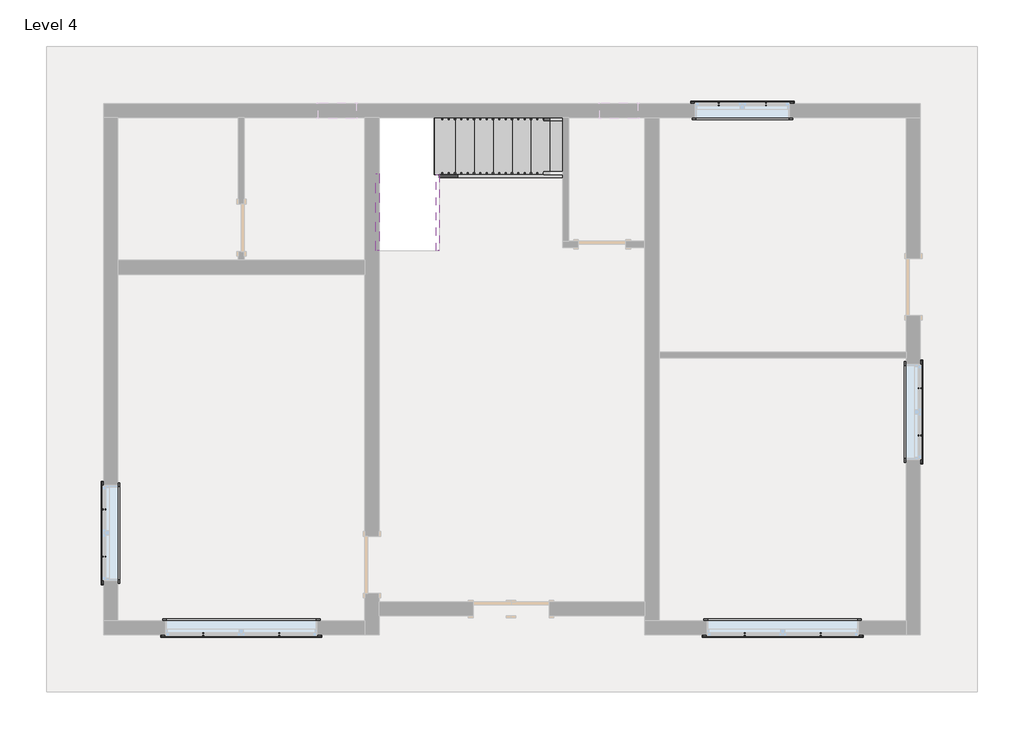
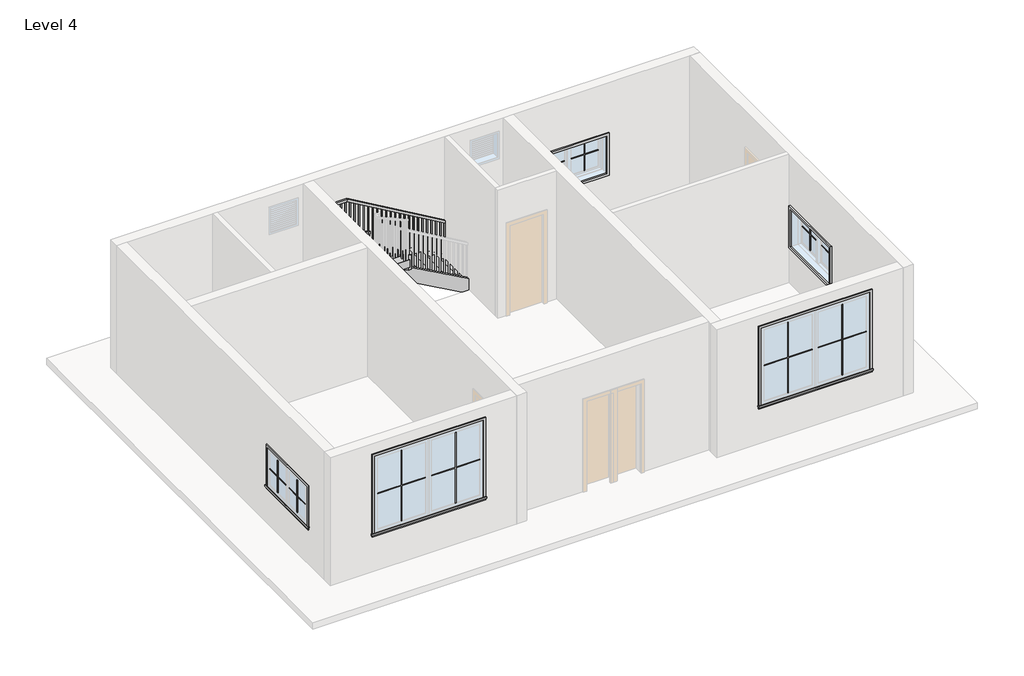
# One storey, part 2 of 2: 20 proxies, 4 members, 1 railing, 1 stair flight.
"""IFC4 building model written with IfcOpenShell, lengths in millimetres."""

from ifc_helpers import new_model, si_unit, frame, origin, place, context, project, spatial, polyline, outline, extrude, faceted_brep, transform, mapped, element, save
from components import muntin_pattern_2x2_muntin_pattern_2x2_9352d081, muntin_pattern_2x2_muntin_pattern_2x2_5c2cbe28, muntin_pattern_2x2_muntin_pattern_2x2_bb8d4d84, muntin_pattern_2x2_muntin_pattern_2x2_d03a1f3c, trim_window_exterior_flat_with_sill_979bde60, trim_window_exterior_flat_with_sill_359ed2ce, trim_window_interior_flat_picture_frame_7883d11b, trim_window_interior_flat_picture_frame_939a8053, stair_flight_aa7d7887

model = new_model("IFC4")

# Units and contexts
model_context = context("Model", 3, world=origin())
ifc_project = project(units=[si_unit("LENGTHUNIT", "METRE", prefix="MILLI")], contexts=[model_context])

# Site, building, storey
site = spatial("IfcSite", under=ifc_project)
building = spatial("IfcBuilding", under=site)
storey = spatial("IfcBuildingStorey", under=building, Name="Level 4", Elevation=9448.8)

# Proxies
placement = place(None, origin())
muntin_pattern_2x2_muntin_pattern_2x2_shape = muntin_pattern_2x2_muntin_pattern_2x2_9352d081(model_context)
element("IfcBuildingElementProxy", 1, Name="Muntin Pattern_2x2 : Muntin Pattern_2x2", ObjectType="Muntin Pattern_2x2 : Muntin Pattern_2x2", at=placement, inside=storey, context=model_context, shape_type="MappedRepresentation", body=[
    mapped(muntin_pattern_2x2_muntin_pattern_2x2_shape, transform((-7798.9165084, -1764.5743005, 10433.05), x_axis=(0.0, 1.0, 0.0), y_axis=(-1.0, 0.0, 0.0), z_axis=(0.0, 0.0, 1.0))),
])
element("IfcBuildingElementProxy", 2, Name="Muntin Pattern_2x2 : Muntin Pattern_2x2", ObjectType="Muntin Pattern_2x2 : Muntin Pattern_2x2", at=placement, inside=storey, context=model_context, shape_type="MappedRepresentation", body=[
    mapped(muntin_pattern_2x2_muntin_pattern_2x2_shape, transform((5288.4334916, 937.3506995, 10433.05), x_axis=(0.0, -1.0, 0.0), y_axis=(1.0, 0.0, 0.0), z_axis=(0.0, 0.0, 1.0))),
])
element("IfcBuildingElementProxy", 3, Name="Muntin Pattern_2x2 : Muntin Pattern_2x2", ObjectType="Muntin Pattern_2x2 : Muntin Pattern_2x2", at=placement, inside=storey, context=model_context, shape_type="MappedRepresentation", body=[
    mapped(muntin_pattern_2x2_muntin_pattern_2x2_shape, transform((2061.0459916, 5501.4131995, 10433.05), x_axis=(1.0, 0.0, 0.0), y_axis=(0.0, 1.0, 0.0), z_axis=(0.0, 0.0, 1.0))),
])
muntin_pattern_2x2_muntin_pattern_2x2_2_shape = muntin_pattern_2x2_muntin_pattern_2x2_5c2cbe28(model_context)
element("IfcBuildingElementProxy", 4, Name="Muntin Pattern_2x2 : Muntin Pattern_2x2", ObjectType="Muntin Pattern_2x2 : Muntin Pattern_2x2", at=placement, inside=storey, context=model_context, shape_type="MappedRepresentation", body=[
    mapped(muntin_pattern_2x2_muntin_pattern_2x2_2_shape, transform((-7798.9165084, -1005.7493005, 10433.05), x_axis=(0.0, -1.0, 0.0), y_axis=(1.0, 0.0, 0.0), z_axis=(0.0, 0.0, 1.0))),
])
element("IfcBuildingElementProxy", 5, Name="Muntin Pattern_2x2 : Muntin Pattern_2x2", ObjectType="Muntin Pattern_2x2 : Muntin Pattern_2x2", at=placement, inside=storey, context=model_context, shape_type="MappedRepresentation", body=[
    mapped(muntin_pattern_2x2_muntin_pattern_2x2_2_shape, transform((5288.4334916, 178.5256995, 10433.05), x_axis=(0.0, 1.0, 0.0), y_axis=(-1.0, 0.0, 0.0), z_axis=(0.0, 0.0, 1.0))),
])
element("IfcBuildingElementProxy", 6, Name="Muntin Pattern_2x2 : Muntin Pattern_2x2", ObjectType="Muntin Pattern_2x2 : Muntin Pattern_2x2", at=placement, inside=storey, context=model_context, shape_type="MappedRepresentation", body=[
    mapped(muntin_pattern_2x2_muntin_pattern_2x2_2_shape, transform((2819.8709916, 5501.4131995, 10433.05), x_axis=(-1.0, 0.0, 0.0), y_axis=(0.0, -1.0, 0.0), z_axis=(0.0, 0.0, 1.0))),
])
muntin_pattern_2x2_muntin_pattern_2x2_3_shape = muntin_pattern_2x2_muntin_pattern_2x2_bb8d4d84(model_context)
element("IfcBuildingElementProxy", 7, Name="Muntin Pattern_2x2 : Muntin Pattern_2x2", ObjectType="Muntin Pattern_2x2 : Muntin Pattern_2x2", at=placement, inside=storey, context=model_context, shape_type="MappedRepresentation", body=[
    mapped(muntin_pattern_2x2_muntin_pattern_2x2_3_shape, transform((-4990.6290084, -3013.9368005, 10433.05), x_axis=(-1.0, 0.0, 0.0), y_axis=(0.0, -1.0, 0.0), z_axis=(0.0, 0.0, 1.0))),
])
element("IfcBuildingElementProxy", 8, Name="Muntin Pattern_2x2 : Muntin Pattern_2x2", ObjectType="Muntin Pattern_2x2 : Muntin Pattern_2x2", at=placement, inside=storey, context=model_context, shape_type="MappedRepresentation", body=[
    mapped(muntin_pattern_2x2_muntin_pattern_2x2_3_shape, transform((3696.1709916, -3013.9368005, 10433.05), x_axis=(-1.0, 0.0, 0.0), y_axis=(0.0, -1.0, 0.0), z_axis=(0.0, 0.0, 1.0))),
])
muntin_pattern_2x2_muntin_pattern_2x2_4_shape = muntin_pattern_2x2_muntin_pattern_2x2_d03a1f3c(model_context)
element("IfcBuildingElementProxy", 9, Name="Muntin Pattern_2x2 : Muntin Pattern_2x2", ObjectType="Muntin Pattern_2x2 : Muntin Pattern_2x2", at=placement, inside=storey, context=model_context, shape_type="MappedRepresentation", body=[
    mapped(muntin_pattern_2x2_muntin_pattern_2x2_4_shape, transform((-6206.6540084, -3013.9368005, 10433.05), x_axis=(1.0, 0.0, 0.0), y_axis=(0.0, 1.0, 0.0), z_axis=(0.0, 0.0, 1.0))),
])
element("IfcBuildingElementProxy", 10, Name="Muntin Pattern_2x2 : Muntin Pattern_2x2", ObjectType="Muntin Pattern_2x2 : Muntin Pattern_2x2", at=placement, inside=storey, context=model_context, shape_type="MappedRepresentation", body=[
    mapped(muntin_pattern_2x2_muntin_pattern_2x2_4_shape, transform((2480.1459916, -3013.9368005, 10433.05), x_axis=(1.0, 0.0, 0.0), y_axis=(0.0, 1.0, 0.0), z_axis=(0.0, 0.0, 1.0))),
])
trim_window_exterior_flat_with_sill_shape = trim_window_exterior_flat_with_sill_979bde60(model_context)
element("IfcBuildingElementProxy", 11, Name="Trim-Window-Exterior-Flat : with Sill", ObjectType="Trim-Window-Exterior-Flat : with Sill", at=placement, inside=storey, context=model_context, shape_type="MappedRepresentation", body=[
    mapped(trim_window_exterior_flat_with_sill_shape, transform((-7808.4415084, -1385.1618005, 11277.6), x_axis=(0.0, -1.0, 0.0), y_axis=(0.0, 0.0, 1.0), z_axis=(-1.0, 0.0, 0.0))),
])
element("IfcBuildingElementProxy", 12, Name="Trim-Window-Exterior-Flat : with Sill", ObjectType="Trim-Window-Exterior-Flat : with Sill", at=placement, inside=storey, context=model_context, shape_type="MappedRepresentation", body=[
    mapped(trim_window_exterior_flat_with_sill_shape, transform((5297.9584916, 557.9381995, 11277.6), x_axis=(0.0, 1.0, 0.0), y_axis=(0.0, 0.0, 1.0), z_axis=(1.0, 0.0, 0.0))),
])
element("IfcBuildingElementProxy", 13, Name="Trim-Window-Exterior-Flat : with Sill", ObjectType="Trim-Window-Exterior-Flat : with Sill", at=placement, inside=storey, context=model_context, shape_type="MappedRepresentation", body=[
    mapped(trim_window_exterior_flat_with_sill_shape, transform((2440.4584916, 5510.9381995, 11277.6), x_axis=(-1.0, 0.0, 0.0), y_axis=(0.0, 0.0, 1.0), z_axis=(0.0, 1.0, 0.0))),
])
trim_window_exterior_flat_with_sill_2_shape = trim_window_exterior_flat_with_sill_359ed2ce(model_context)
element("IfcBuildingElementProxy", 14, Name="Trim-Window-Exterior-Flat : with Sill", ObjectType="Trim-Window-Exterior-Flat : with Sill", at=placement, inside=storey, context=model_context, shape_type="MappedRepresentation", body=[
    mapped(trim_window_exterior_flat_with_sill_2_shape, transform((-5598.6415084, -3023.4618005, 12192.0), x_axis=(1.0, 0.0, 0.0), y_axis=(0.0, 0.0, 1.0), z_axis=(0.0, -1.0, 0.0))),
])
element("IfcBuildingElementProxy", 15, Name="Trim-Window-Exterior-Flat : with Sill", ObjectType="Trim-Window-Exterior-Flat : with Sill", at=placement, inside=storey, context=model_context, shape_type="MappedRepresentation", body=[
    mapped(trim_window_exterior_flat_with_sill_2_shape, transform((3088.1584916, -3023.4618005, 12192.0), x_axis=(1.0, 0.0, 0.0), y_axis=(0.0, 0.0, 1.0), z_axis=(0.0, -1.0, 0.0))),
])
trim_window_interior_flat_picture_frame_shape = trim_window_interior_flat_picture_frame_7883d11b(model_context)
element("IfcBuildingElementProxy", 16, Name="Trim-Window-Interior-Flat : Picture Frame", ObjectType="Trim-Window-Interior-Flat : Picture Frame", at=placement, inside=storey, context=model_context, shape_type="MappedRepresentation", body=[
    mapped(trim_window_interior_flat_picture_frame_shape, transform((-7579.8415084, -1385.1618005, 11277.6), x_axis=(0.0, 1.0, 0.0), y_axis=(0.0, 0.0, 1.0), z_axis=(1.0, 0.0, 0.0))),
])
element("IfcBuildingElementProxy", 17, Name="Trim-Window-Interior-Flat : Picture Frame", ObjectType="Trim-Window-Interior-Flat : Picture Frame", at=placement, inside=storey, context=model_context, shape_type="MappedRepresentation", body=[
    mapped(trim_window_interior_flat_picture_frame_shape, transform((5069.3584916, 557.9381995, 11277.6), x_axis=(0.0, -1.0, 0.0), y_axis=(0.0, 0.0, 1.0), z_axis=(-1.0, 0.0, 0.0))),
])
element("IfcBuildingElementProxy", 18, Name="Trim-Window-Interior-Flat : Picture Frame", ObjectType="Trim-Window-Interior-Flat : Picture Frame", at=placement, inside=storey, context=model_context, shape_type="MappedRepresentation", body=[
    mapped(trim_window_interior_flat_picture_frame_shape, transform((2440.4584916, 5282.3381995, 11277.6), x_axis=(1.0, 0.0, 0.0), y_axis=(0.0, 0.0, 1.0), z_axis=(0.0, -1.0, 0.0))),
])
trim_window_interior_flat_picture_frame_2_shape = trim_window_interior_flat_picture_frame_939a8053(model_context)
element("IfcBuildingElementProxy", 19, Name="Trim-Window-Interior-Flat : Picture Frame", ObjectType="Trim-Window-Interior-Flat : Picture Frame", at=placement, inside=storey, context=model_context, shape_type="MappedRepresentation", body=[
    mapped(trim_window_interior_flat_picture_frame_2_shape, transform((-5598.6415084, -2794.8618005, 12192.0), x_axis=(-1.0, 0.0, 0.0), y_axis=(0.0, 0.0, 1.0), z_axis=(0.0, 1.0, 0.0))),
])
element("IfcBuildingElementProxy", 20, Name="Trim-Window-Interior-Flat : Picture Frame", ObjectType="Trim-Window-Interior-Flat : Picture Frame", at=placement, inside=storey, context=model_context, shape_type="MappedRepresentation", body=[
    mapped(trim_window_interior_flat_picture_frame_2_shape, transform((3088.1584916, -2794.8618005, 12192.0), x_axis=(-1.0, 0.0, 0.0), y_axis=(0.0, 0.0, 1.0), z_axis=(0.0, 1.0, 0.0))),
])

# Members
element("IfcMember", 21, ObjectType="Stringer - 2\" Width", at=placement, inside=storey, context=model_context, shape_type="SweptSolid", body=[
    extrude(outline(polyline([(9448.8, -442.4415084), (9712.8428392, -442.4415084), (10813.5095059, -2423.6415084), (10464.8308318, -2423.6415084), (9448.8, -594.7860112), (9448.8, -442.4415084)])), frame((0.0, 4317.5146777, 0.0), z_axis=(0.0, 1.0, 0.0), x_axis=(0.0, 0.0, 1.0)), (0.0, 0.0, 1.0), 50.8),
])
element("IfcMember", 22, ObjectType="Stringer - 2\" Width", at=placement, inside=storey, context=model_context, shape_type="SweptSolid", body=[
    extrude(outline(polyline([(4368.3146777, 11011.045537), (4368.3146777, 10662.4006925), (3148.7383287, 11339.6643411), (3148.7383287, 11688.3091856), (4368.3146777, 11011.045537)])), frame((-2474.4415084, 0.0, 0.0), z_axis=(1.0, 0.0, 0.0), x_axis=(0.0, 1.0, 0.0)), (0.0, 0.0, 1.0), 50.8),
])
element("IfcMember", 23, ObjectType="Stringer - 2\" Width", at=placement, inside=storey, context=model_context, shape_type="SweptSolid", body=[
    extrude(outline(polyline([(9448.8, -442.4415084), (9712.8428392, -442.4415084), (10503.4636166, -1865.5589077), (10503.4636166, -2493.1805211), (9448.8, -594.7860112), (9448.8, -442.4415084)])), frame((0.0, 5282.3381995, 0.0), z_axis=(0.0, 1.0, 0.0), x_axis=(0.0, 0.0, 1.0)), (0.0, 0.0, 1.0), 50.8),
])
element("IfcMember", 24, ObjectType="Stringer - 2\" Width", at=placement, inside=storey, context=model_context, shape_type="SweptSolid", body=[
    extrude(outline(polyline([(3758.489521, 11001.053054), (3148.7383287, 11339.6643411), (3148.7383287, 11688.3091856), (4386.3085505, 11001.053054), (3758.489521, 11001.053054)])), frame((-3439.6415084, 0.0, 0.0), z_axis=(1.0, 0.0, 0.0), x_axis=(0.0, 1.0, 0.0)), (0.0, 0.0, 1.0), 50.8),
])

# Railing
element("IfcRailing", 25, ObjectType="Handrail - Rectangular", at=placement, inside=storey, context=model_context, shape_type="SolidModel", body=[
    faceted_brep([(-442.4415084, 5231.5381995, 10532.5333333), (-442.4415084, 5231.5381995, 10473.7219871), (-442.4415084, 5282.3381995, 10473.7219871), (-442.4415084, 5282.3381995, 10532.5333333), (-2641.0608886, 5231.5381995, 11815.0613051), (-2654.794625, 5231.5381995, 11764.2613051), (-2654.794625, 5282.3381995, 11764.2613051), (-2641.0608886, 5282.3381995, 11815.0613051), (-3338.0415084, 5231.5381995, 11815.0613051), (-3338.0415084, 5231.5381995, 11764.2613051), (-3388.8415084, 5282.3381995, 11764.2613051), (-3388.8415084, 5282.3381995, 11815.0613051), (-3338.0415084, 4498.2044111, 11815.0613051), (-3338.0415084, 4485.04436, 11764.2613051), (-3388.8415084, 4485.04436, 11764.2613051), (-3388.8415084, 4498.2044111, 11815.0613051), (-3338.0415084, 3148.7383287, 12564.5333333), (-3388.8415084, 3148.7383287, 12564.5333333), (-3388.8415084, 3148.7383287, 12506.42445), (-3338.0415084, 3148.7383287, 12506.42445)], [[[0, 1, 2, 3]], [[1, 0, 4, 5]], [[2, 1, 5, 6]], [[3, 2, 6, 7]], [[0, 3, 7, 4]], [[5, 4, 8, 9]], [[6, 5, 9, 10]], [[7, 6, 10, 11]], [[4, 7, 11, 8]], [[9, 8, 12, 13]], [[10, 9, 13, 14]], [[11, 10, 14, 15]], [[8, 11, 15, 12]], [[16, 17, 18, 19]], [[13, 12, 16, 19]], [[14, 13, 19, 18]], [[15, 14, 18, 17]], [[12, 15, 17, 16]]]),
    extrude(outline(polyline([(3215.4131995, 12469.3942858), (3234.4631995, 12458.8142183), (3234.4631995, 11480.8), (3215.4131995, 11480.8), (3215.4131995, 12469.3942858)])), frame((-3372.9665084, 0.0, 0.0), z_axis=(1.0, 0.0, 0.0), x_axis=(0.0, 1.0, 0.0)), (0.0, 0.0, 1.0), 19.05),
    extrude(outline(polyline([(3317.0131995, 12413.1240232), (3336.0631995, 12402.5439558), (3336.0631995, 11480.8), (3317.0131995, 11480.8), (3317.0131995, 12413.1240232)])), frame((-3372.9665084, 0.0, 0.0), z_axis=(1.0, 0.0, 0.0), x_axis=(0.0, 1.0, 0.0)), (0.0, 0.0, 1.0), 19.05),
    extrude(outline(polyline([(3418.6131995, 12356.6969969), (3437.6631995, 12346.1169295), (3437.6631995, 11480.8), (3418.6131995, 11480.8), (3418.6131995, 12356.6969969)])), frame((-3372.9665084, 0.0, 0.0), z_axis=(1.0, 0.0, 0.0), x_axis=(0.0, 1.0, 0.0)), (0.0, 0.0, 1.0), 19.05),
    extrude(outline(polyline([(3520.2131995, 12300.2699707), (3539.2631995, 12289.6899033), (3539.2631995, 11311.4666667), (3520.2131995, 11311.4666667), (3520.2131995, 12300.2699707)])), frame((-3372.9665084, 0.0, 0.0), z_axis=(1.0, 0.0, 0.0), x_axis=(0.0, 1.0, 0.0)), (0.0, 0.0, 1.0), 19.05),
    extrude(outline(polyline([(3621.8131995, 12243.7906899), (3640.8631995, 12233.2106224), (3640.8631995, 11311.4666667), (3621.8131995, 11311.4666667), (3621.8131995, 12243.7906899)])), frame((-3372.9665084, 0.0, 0.0), z_axis=(1.0, 0.0, 0.0), x_axis=(0.0, 1.0, 0.0)), (0.0, 0.0, 1.0), 19.05),
    extrude(outline(polyline([(3723.4131995, 12187.3636636), (3742.4631995, 12176.7835962), (3742.4631995, 11311.4666667), (3723.4131995, 11311.4666667), (3723.4131995, 12187.3636636)])), frame((-3372.9665084, 0.0, 0.0), z_axis=(1.0, 0.0, 0.0), x_axis=(0.0, 1.0, 0.0)), (0.0, 0.0, 1.0), 19.05),
    extrude(outline(polyline([(3825.0131995, 12130.9366374), (3844.0631995, 12120.3565699), (3844.0631995, 11142.1333333), (3825.0131995, 11142.1333333), (3825.0131995, 12130.9366374)])), frame((-3372.9665084, 0.0, 0.0), z_axis=(1.0, 0.0, 0.0), x_axis=(0.0, 1.0, 0.0)), (0.0, 0.0, 1.0), 19.05),
    extrude(outline(polyline([(3926.6131995, 12074.4573565), (3945.6631995, 12063.8772891), (3945.6631995, 11142.1333333), (3926.6131995, 11142.1333333), (3926.6131995, 12074.4573565)])), frame((-3372.9665084, 0.0, 0.0), z_axis=(1.0, 0.0, 0.0), x_axis=(0.0, 1.0, 0.0)), (0.0, 0.0, 1.0), 19.05),
    extrude(outline(polyline([(4028.2131995, 12018.0303303), (4047.2631995, 12007.4502629), (4047.2631995, 11142.1333333), (4028.2131995, 11142.1333333), (4028.2131995, 12018.0303303)])), frame((-3372.9665084, 0.0, 0.0), z_axis=(1.0, 0.0, 0.0), x_axis=(0.0, 1.0, 0.0)), (0.0, 0.0, 1.0), 19.05),
    extrude(outline(polyline([(4129.8131995, 11961.603304), (4148.8631995, 11951.0232366), (4148.8631995, 10972.8), (4129.8131995, 10972.8), (4129.8131995, 11961.603304)])), frame((-3372.9665084, 0.0, 0.0), z_axis=(1.0, 0.0, 0.0), x_axis=(0.0, 1.0, 0.0)), (0.0, 0.0, 1.0), 19.05),
    extrude(outline(polyline([(4231.4131995, 11905.1240232), (4250.4631995, 11894.5439558), (4250.4631995, 10972.8), (4231.4131995, 10972.8), (4231.4131995, 11905.1240232)])), frame((-3372.9665084, 0.0, 0.0), z_axis=(1.0, 0.0, 0.0), x_axis=(0.0, 1.0, 0.0)), (0.0, 0.0, 1.0), 19.05),
    extrude(outline(polyline([(4333.0131995, 11848.6969969), (4352.0631995, 11838.1169295), (4352.0631995, 10972.8), (4333.0131995, 10972.8), (4333.0131995, 11848.6969969)])), frame((-3372.9665084, 0.0, 0.0), z_axis=(1.0, 0.0, 0.0), x_axis=(0.0, 1.0, 0.0)), (0.0, 0.0, 1.0), 19.05),
    extrude(outline(polyline([(4434.6131995, 11792.2699707), (4453.6631995, 11781.6899033), (4453.6631995, 10803.4666667), (4434.6131995, 10803.4666667), (4434.6131995, 11792.2699707)])), frame((-3372.9665084, 0.0, 0.0), z_axis=(1.0, 0.0, 0.0), x_axis=(0.0, 1.0, 0.0)), (0.0, 0.0, 1.0), 19.05),
    extrude(outline(polyline([(-3372.9665084, 4555.2631995), (-3353.9165084, 4555.2631995), (-3353.9165084, 4536.2131995), (-3372.9665084, 4536.2131995), (-3372.9665084, 4555.2631995)])), frame((0.0, 0.0, 10803.4666667), z_axis=(0.0, 0.0, 1.0), x_axis=(1.0, 0.0, 0.0)), (0.0, 0.0, 1.0), 960.7946385),
    extrude(outline(polyline([(-3372.9665084, 4656.8631995), (-3353.9165084, 4656.8631995), (-3353.9165084, 4637.8131995), (-3372.9665084, 4637.8131995), (-3372.9665084, 4656.8631995)])), frame((0.0, 0.0, 10803.4666667), z_axis=(0.0, 0.0, 1.0), x_axis=(1.0, 0.0, 0.0)), (0.0, 0.0, 1.0), 960.7946385),
    extrude(outline(polyline([(-3372.9665084, 4758.4631995), (-3353.9165084, 4758.4631995), (-3353.9165084, 4739.4131995), (-3372.9665084, 4739.4131995), (-3372.9665084, 4758.4631995)])), frame((0.0, 0.0, 10803.4666667), z_axis=(0.0, 0.0, 1.0), x_axis=(1.0, 0.0, 0.0)), (0.0, 0.0, 1.0), 960.7946385),
    extrude(outline(polyline([(-3372.9665084, 4860.0631995), (-3353.9165084, 4860.0631995), (-3353.9165084, 4841.0131995), (-3372.9665084, 4841.0131995), (-3372.9665084, 4860.0631995)])), frame((0.0, 0.0, 10803.4666667), z_axis=(0.0, 0.0, 1.0), x_axis=(1.0, 0.0, 0.0)), (0.0, 0.0, 1.0), 960.7946385),
    extrude(outline(polyline([(-3372.9665084, 4961.6631995), (-3353.9165084, 4961.6631995), (-3353.9165084, 4942.6131995), (-3372.9665084, 4942.6131995), (-3372.9665084, 4961.6631995)])), frame((0.0, 0.0, 10803.4666667), z_axis=(0.0, 0.0, 1.0), x_axis=(1.0, 0.0, 0.0)), (0.0, 0.0, 1.0), 960.7946385),
    extrude(outline(polyline([(-3372.9665084, 5063.2631995), (-3353.9165084, 5063.2631995), (-3353.9165084, 5044.2131995), (-3372.9665084, 5044.2131995), (-3372.9665084, 5063.2631995)])), frame((0.0, 0.0, 10803.4666667), z_axis=(0.0, 0.0, 1.0), x_axis=(1.0, 0.0, 0.0)), (0.0, 0.0, 1.0), 960.7946385),
    extrude(outline(polyline([(-3372.9665084, 5164.8631995), (-3353.9165084, 5164.8631995), (-3353.9165084, 5145.8131995), (-3372.9665084, 5145.8131995), (-3372.9665084, 5164.8631995)])), frame((0.0, 0.0, 10803.4666667), z_axis=(0.0, 0.0, 1.0), x_axis=(1.0, 0.0, 0.0)), (0.0, 0.0, 1.0), 960.7946385),
    extrude(outline(polyline([(-3277.7165084, 5266.4631995), (-3277.7165084, 5247.4131995), (-3296.7665084, 5247.4131995), (-3296.7665084, 5266.4631995), (-3277.7165084, 5266.4631995)])), frame((0.0, 0.0, 10803.4666667), z_axis=(0.0, 0.0, 1.0), x_axis=(1.0, 0.0, 0.0)), (0.0, 0.0, 1.0), 960.7946385),
    extrude(outline(polyline([(-3176.1165084, 5266.4631995), (-3176.1165084, 5247.4131995), (-3195.1665084, 5247.4131995), (-3195.1665084, 5266.4631995), (-3176.1165084, 5266.4631995)])), frame((0.0, 0.0, 10803.4666667), z_axis=(0.0, 0.0, 1.0), x_axis=(1.0, 0.0, 0.0)), (0.0, 0.0, 1.0), 960.7946385),
    extrude(outline(polyline([(-3074.5165084, 5266.4631995), (-3074.5165084, 5247.4131995), (-3093.5665084, 5247.4131995), (-3093.5665084, 5266.4631995), (-3074.5165084, 5266.4631995)])), frame((0.0, 0.0, 10803.4666667), z_axis=(0.0, 0.0, 1.0), x_axis=(1.0, 0.0, 0.0)), (0.0, 0.0, 1.0), 960.7946385),
    extrude(outline(polyline([(-2972.9165084, 5266.4631995), (-2972.9165084, 5247.4131995), (-2991.9665084, 5247.4131995), (-2991.9665084, 5266.4631995), (-2972.9165084, 5266.4631995)])), frame((0.0, 0.0, 10803.4666667), z_axis=(0.0, 0.0, 1.0), x_axis=(1.0, 0.0, 0.0)), (0.0, 0.0, 1.0), 960.7946385),
    extrude(outline(polyline([(-2871.3165084, 5266.4631995), (-2871.3165084, 5247.4131995), (-2890.3665084, 5247.4131995), (-2890.3665084, 5266.4631995), (-2871.3165084, 5266.4631995)])), frame((0.0, 0.0, 10803.4666667), z_axis=(0.0, 0.0, 1.0), x_axis=(1.0, 0.0, 0.0)), (0.0, 0.0, 1.0), 960.7946385),
    extrude(outline(polyline([(-2769.7165084, 5266.4631995), (-2769.7165084, 5247.4131995), (-2788.7665084, 5247.4131995), (-2788.7665084, 5266.4631995), (-2769.7165084, 5266.4631995)])), frame((0.0, 0.0, 10803.4666667), z_axis=(0.0, 0.0, 1.0), x_axis=(1.0, 0.0, 0.0)), (0.0, 0.0, 1.0), 960.7946385),
    extrude(outline(polyline([(-2668.1165084, 5266.4631995), (-2668.1165084, 5247.4131995), (-2687.1665084, 5247.4131995), (-2687.1665084, 5266.4631995), (-2668.1165084, 5266.4631995)])), frame((0.0, 0.0, 10803.4666667), z_axis=(0.0, 0.0, 1.0), x_axis=(1.0, 0.0, 0.0)), (0.0, 0.0, 1.0), 960.7946385),
    extrude(outline(polyline([(11712.7657371, -2566.5165084), (11723.8782371, -2585.5665084), (10803.4666667, -2585.5665084), (10803.4666667, -2566.5165084), (11712.7657371, -2566.5165084)])), frame((0.0, 5247.4131995, 0.0), z_axis=(0.0, 1.0, 0.0), x_axis=(0.0, 0.0, 1.0)), (0.0, 0.0, 1.0), 19.05),
    extrude(outline(polyline([(11653.4990704, -2464.9165084), (11664.6115704, -2483.9665084), (10803.4666667, -2483.9665084), (10803.4666667, -2464.9165084), (11653.4990704, -2464.9165084)])), frame((0.0, 5247.4131995, 0.0), z_axis=(0.0, 1.0, 0.0), x_axis=(0.0, 0.0, 1.0)), (0.0, 0.0, 1.0), 19.05),
    extrude(outline(polyline([(11594.2324038, -2363.3165084), (11605.3449038, -2382.3665084), (10634.1333333, -2382.3665084), (10634.1333333, -2363.3165084), (11594.2324038, -2363.3165084)])), frame((0.0, 5247.4131995, 0.0), z_axis=(0.0, 1.0, 0.0), x_axis=(0.0, 0.0, 1.0)), (0.0, 0.0, 1.0), 19.05),
    extrude(outline(polyline([(11534.9657371, -2261.7165084), (11546.0782371, -2280.7665084), (10634.1333333, -2280.7665084), (10634.1333333, -2261.7165084), (11534.9657371, -2261.7165084)])), frame((0.0, 5247.4131995, 0.0), z_axis=(0.0, 1.0, 0.0), x_axis=(0.0, 0.0, 1.0)), (0.0, 0.0, 1.0), 19.05),
    extrude(outline(polyline([(11475.6990704, -2160.1165084), (11486.8115704, -2179.1665084), (10634.1333333, -2179.1665084), (10634.1333333, -2160.1165084), (11475.6990704, -2160.1165084)])), frame((0.0, 5247.4131995, 0.0), z_axis=(0.0, 1.0, 0.0), x_axis=(0.0, 0.0, 1.0)), (0.0, 0.0, 1.0), 19.05),
    extrude(outline(polyline([(11416.4324038, -2058.5165084), (11427.5449038, -2077.5665084), (10464.8, -2077.5665084), (10464.8, -2058.5165084), (11416.4324038, -2058.5165084)])), frame((0.0, 5247.4131995, 0.0), z_axis=(0.0, 1.0, 0.0), x_axis=(0.0, 0.0, 1.0)), (0.0, 0.0, 1.0), 19.05),
    extrude(outline(polyline([(11357.1657371, -1956.9165084), (11368.2782371, -1975.9665084), (10464.8, -1975.9665084), (10464.8, -1956.9165084), (11357.1657371, -1956.9165084)])), frame((0.0, 5247.4131995, 0.0), z_axis=(0.0, 1.0, 0.0), x_axis=(0.0, 0.0, 1.0)), (0.0, 0.0, 1.0), 19.05),
    extrude(outline(polyline([(11297.8990704, -1855.3165084), (11309.0115704, -1874.3665084), (10464.8, -1874.3665084), (10464.8, -1855.3165084), (11297.8990704, -1855.3165084)])), frame((0.0, 5247.4131995, 0.0), z_axis=(0.0, 1.0, 0.0), x_axis=(0.0, 0.0, 1.0)), (0.0, 0.0, 1.0), 19.05),
    extrude(outline(polyline([(11238.6324038, -1753.7165084), (11249.7449038, -1772.7665084), (10295.4666667, -1772.7665084), (10295.4666667, -1753.7165084), (11238.6324038, -1753.7165084)])), frame((0.0, 5247.4131995, 0.0), z_axis=(0.0, 1.0, 0.0), x_axis=(0.0, 0.0, 1.0)), (0.0, 0.0, 1.0), 19.05),
    extrude(outline(polyline([(11179.3657371, -1652.1165084), (11190.4782371, -1671.1665084), (10295.4666667, -1671.1665084), (10295.4666667, -1652.1165084), (11179.3657371, -1652.1165084)])), frame((0.0, 5247.4131995, 0.0), z_axis=(0.0, 1.0, 0.0), x_axis=(0.0, 0.0, 1.0)), (0.0, 0.0, 1.0), 19.05),
    extrude(outline(polyline([(11120.0990704, -1550.5165084), (11131.2115704, -1569.5665084), (10295.4666667, -1569.5665084), (10295.4666667, -1550.5165084), (11120.0990704, -1550.5165084)])), frame((0.0, 5247.4131995, 0.0), z_axis=(0.0, 1.0, 0.0), x_axis=(0.0, 0.0, 1.0)), (0.0, 0.0, 1.0), 19.05),
    extrude(outline(polyline([(11060.8324038, -1448.9165084), (11071.9449038, -1467.9665084), (10126.1333333, -1467.9665084), (10126.1333333, -1448.9165084), (11060.8324038, -1448.9165084)])), frame((0.0, 5247.4131995, 0.0), z_axis=(0.0, 1.0, 0.0), x_axis=(0.0, 0.0, 1.0)), (0.0, 0.0, 1.0), 19.05),
    extrude(outline(polyline([(11001.5657371, -1347.3165084), (11012.6782371, -1366.3665084), (10126.1333333, -1366.3665084), (10126.1333333, -1347.3165084), (11001.5657371, -1347.3165084)])), frame((0.0, 5247.4131995, 0.0), z_axis=(0.0, 1.0, 0.0), x_axis=(0.0, 0.0, 1.0)), (0.0, 0.0, 1.0), 19.05),
    extrude(outline(polyline([(10942.2990704, -1245.7165084), (10953.4115704, -1264.7665084), (10126.1333333, -1264.7665084), (10126.1333333, -1245.7165084), (10942.2990704, -1245.7165084)])), frame((0.0, 5247.4131995, 0.0), z_axis=(0.0, 1.0, 0.0), x_axis=(0.0, 0.0, 1.0)), (0.0, 0.0, 1.0), 19.05),
    extrude(outline(polyline([(10883.0324038, -1144.1165084), (10894.1449038, -1163.1665084), (9956.8, -1163.1665084), (9956.8, -1144.1165084), (10883.0324038, -1144.1165084)])), frame((0.0, 5247.4131995, 0.0), z_axis=(0.0, 1.0, 0.0), x_axis=(0.0, 0.0, 1.0)), (0.0, 0.0, 1.0), 19.05),
    extrude(outline(polyline([(10823.7657371, -1042.5165084), (10834.8782371, -1061.5665084), (9956.8, -1061.5665084), (9956.8, -1042.5165084), (10823.7657371, -1042.5165084)])), frame((0.0, 5247.4131995, 0.0), z_axis=(0.0, 1.0, 0.0), x_axis=(0.0, 0.0, 1.0)), (0.0, 0.0, 1.0), 19.05),
    extrude(outline(polyline([(10764.4990704, -940.9165084), (10775.6115704, -959.9665084), (9956.8, -959.9665084), (9956.8, -940.9165084), (10764.4990704, -940.9165084)])), frame((0.0, 5247.4131995, 0.0), z_axis=(0.0, 1.0, 0.0), x_axis=(0.0, 0.0, 1.0)), (0.0, 0.0, 1.0), 19.05),
    extrude(outline(polyline([(10705.2324038, -839.3165084), (10716.3449038, -858.3665084), (9787.4666667, -858.3665084), (9787.4666667, -839.3165084), (10705.2324038, -839.3165084)])), frame((0.0, 5247.4131995, 0.0), z_axis=(0.0, 1.0, 0.0), x_axis=(0.0, 0.0, 1.0)), (0.0, 0.0, 1.0), 19.05),
    extrude(outline(polyline([(10645.9657371, -737.7165084), (10657.0782371, -756.7665084), (9787.4666667, -756.7665084), (9787.4666667, -737.7165084), (10645.9657371, -737.7165084)])), frame((0.0, 5247.4131995, 0.0), z_axis=(0.0, 1.0, 0.0), x_axis=(0.0, 0.0, 1.0)), (0.0, 0.0, 1.0), 19.05),
    extrude(outline(polyline([(10586.6990704, -636.1165084), (10597.8115704, -655.1665084), (9787.4666667, -655.1665084), (9787.4666667, -636.1165084), (10586.6990704, -636.1165084)])), frame((0.0, 5247.4131995, 0.0), z_axis=(0.0, 1.0, 0.0), x_axis=(0.0, 0.0, 1.0)), (0.0, 0.0, 1.0), 19.05),
    extrude(outline(polyline([(10527.4324038, -534.5165084), (10538.5449038, -553.5665084), (9618.1333333, -553.5665084), (9618.1333333, -534.5165084), (10527.4324038, -534.5165084)])), frame((0.0, 5247.4131995, 0.0), z_axis=(0.0, 1.0, 0.0), x_axis=(0.0, 0.0, 1.0)), (0.0, 0.0, 1.0), 19.05),
    extrude(outline(polyline([(-3353.9165084, 5266.4631995), (-3353.9165084, 5247.4131995), (-3372.9665084, 5247.4131995), (-3372.9665084, 5266.4631995), (-3353.9165084, 5266.4631995)])), frame((0.0, 0.0, 10803.4666667), z_axis=(0.0, 0.0, 1.0), x_axis=(1.0, 0.0, 0.0)), (0.0, 0.0, 1.0), 960.7946385),
    extrude(outline(polyline([(3148.7383287, 12506.42445), (3167.7883287, 12495.8443826), (3167.7883287, 11480.8), (3148.7383287, 11480.8), (3148.7383287, 12506.42445)])), frame((-3372.9665084, 0.0, 0.0), z_axis=(1.0, 0.0, 0.0), x_axis=(0.0, 1.0, 0.0)), (0.0, 0.0, 1.0), 19.05),
    extrude(outline(polyline([(10473.7219871, -442.4415084), (10484.8344871, -461.4915084), (9618.1333333, -461.4915084), (9618.1333333, -442.4415084), (10473.7219871, -442.4415084)])), frame((0.0, 5247.4131995, 0.0), z_axis=(0.0, 1.0, 0.0), x_axis=(0.0, 0.0, 1.0)), (0.0, 0.0, 1.0), 19.05),
])

# Stair flight
stair_flight_shape = stair_flight_aa7d7887(model_context)
element("IfcStairFlight", 26, ObjectType="2\" Tread 1\" Nosing 1/4\" Riser", at=placement, inside=storey, context=model_context, shape_type="MappedRepresentation", body=[
    mapped(stair_flight_shape, transform((0.0, 0.0, 0.0), x_axis=(1.0, 0.0, 0.0), y_axis=(0.0, 1.0, 0.0), z_axis=(0.0, 0.0, 1.0))),
])

save(model, "model.ifc")

# Revit data of these elements
# Type "Muntin Pattern_2x2 : Muntin Pattern_2x2"
#   Width [instance default] = 4' - 0"
#   Thickness = 0' - 0 1/2"
#   Height [instance default] = 4' - 0"
#   Distance = 0' - 0 3/4"
#   Interior Material [instance default] = none
#   Exterior Material [instance default] = none
#   Default Elevation = 0
# Type "Trim-Window-Exterior-Flat : with Sill"
#   Trim Width = 0' - 2 1/4"
#   Trim Thickness_Picture Frame = 0' - 1 1/4"
#   Trim Thickness_with Sill = 0' - 0 3/4"
#   Sill Thickness = 0' - 1 1/4"
#   Opening Width [instance default] = 2' - 0"
#   Opening Height [instance default] = 3' - 0"
#   Default Elevation = 4' - 0"
#   Sill = yes
#   Picture Frame = no
#   Trim Material [instance default] = none
# Type "Trim-Window-Interior-Flat : Picture Frame"
#   Trim Thickness_Picture Frame = 0' - 1 1/4"
#   Trim Width = 0' - 2 1/4"
#   Trim Thickness_with Sill = 0' - 0 3/4"
#   Sill Thickness = 0' - 1 1/4"
#   Opening Width [instance default] = 2' - 0"
#   Opening Height [instance default] = 3' - 0"
#   Default Elevation = 4' - 0"
#   Sill = no
#   Picture Frame = yes
#   Trim Material [instance default] = none
# Type "Handrail - Rectangular"
#   Assembly Code = "C2010400"
#   built-in parameter 1008612 = 0.0416667 (stored number, unit not read)
#   built-in parameter 1008611 = 0.0416667 (stored number, unit not read)
#   built-in parameter 1008609 = 0.333333 (stored number, unit not read)
#   built-in parameter 1008604 = 0.166667 (stored number, unit not read)
#   built-in parameter 1008603 = 0.166667 (stored number, unit not read)
#   Railing Height = 3' - 0"
#   built-in parameter 1008630 = 2
#   built-in parameter 1008610 = 2
#   built-in parameter 1008618 = Baluster - Square : 3/4"
# Elements 1, 2, 3, 4, 5, 6 (IfcBuildingElementProxy, "Muntin Pattern_2x2 : Muntin Pattern_2x2")
#   Width = 2' - 0 5/8"
#   Height = 2' - 6 1/2"
#   Interior Material = Wood - Stained
#   Exterior Material = Clad - White
#   Phase Created = New Construction
#   Materials on its faces: "Clad - White", "Wood - Stained"
# Elements 7, 8, 9, 10 (IfcBuildingElementProxy, "Muntin Pattern_2x2 : Muntin Pattern_2x2")
#   Width = 3' - 6 5/8"
#   Height = 5' - 6 1/2"
#   Interior Material = Wood - Stained
#   Exterior Material = Clad - White
#   Phase Created = New Construction
#   Materials on its faces: "Clad - White", "Wood - Stained"
# Elements 11, 12, 13 (IfcBuildingElementProxy, "Trim-Window-Exterior-Flat : with Sill")
#   Opening Width = 5' - 0"
#   Opening Height = 3' - 0"
#   Trim Material = Clad - White
#   Phase Created = New Construction
#   Materials on its faces: "Clad - White"
# Elements 14, 15 (IfcBuildingElementProxy, "Trim-Window-Exterior-Flat : with Sill")
#   Opening Width = 8' - 0"
#   Opening Height = 6' - 0"
#   Trim Material = Clad - White
#   Phase Created = New Construction
#   Materials on its faces: "Clad - White"
# Elements 16, 17, 18 (IfcBuildingElementProxy, "Trim-Window-Interior-Flat : Picture Frame")
#   Opening Width = 5' - 0"
#   Opening Height = 3' - 0"
#   Trim Material = Wood - Stained
#   Phase Created = New Construction
#   Materials on its faces: "Wood - Stained"
# Elements 19, 20 (IfcBuildingElementProxy, "Trim-Window-Interior-Flat : Picture Frame")
#   Opening Width = 8' - 0"
#   Opening Height = 6' - 0"
#   Trim Material = Wood - Stained
#   Phase Created = New Construction
#   Materials on its faces: "Wood - Stained"
# Elements 21, 22, 23, 24 (IfcMember, "Stringer - 2\" Width")
#   Phase Created = New Construction
# Element 25 (IfcRailing, "Handrail - Rectangular")
#   Phase Created = New Construction
# Element 26 (IfcStairFlight, "2\" Tread 1\" Nosing 1/4\" Riser")
#   Phase Created = New Construction
# Materials
#   "Clad - White": class "Wood", colour RGB 242 242 238, transparency 0, Cost = 0
#   "Wood - Stained": class "Wood", colour RGB 224 178 126, transparency 0, Cost = 0
